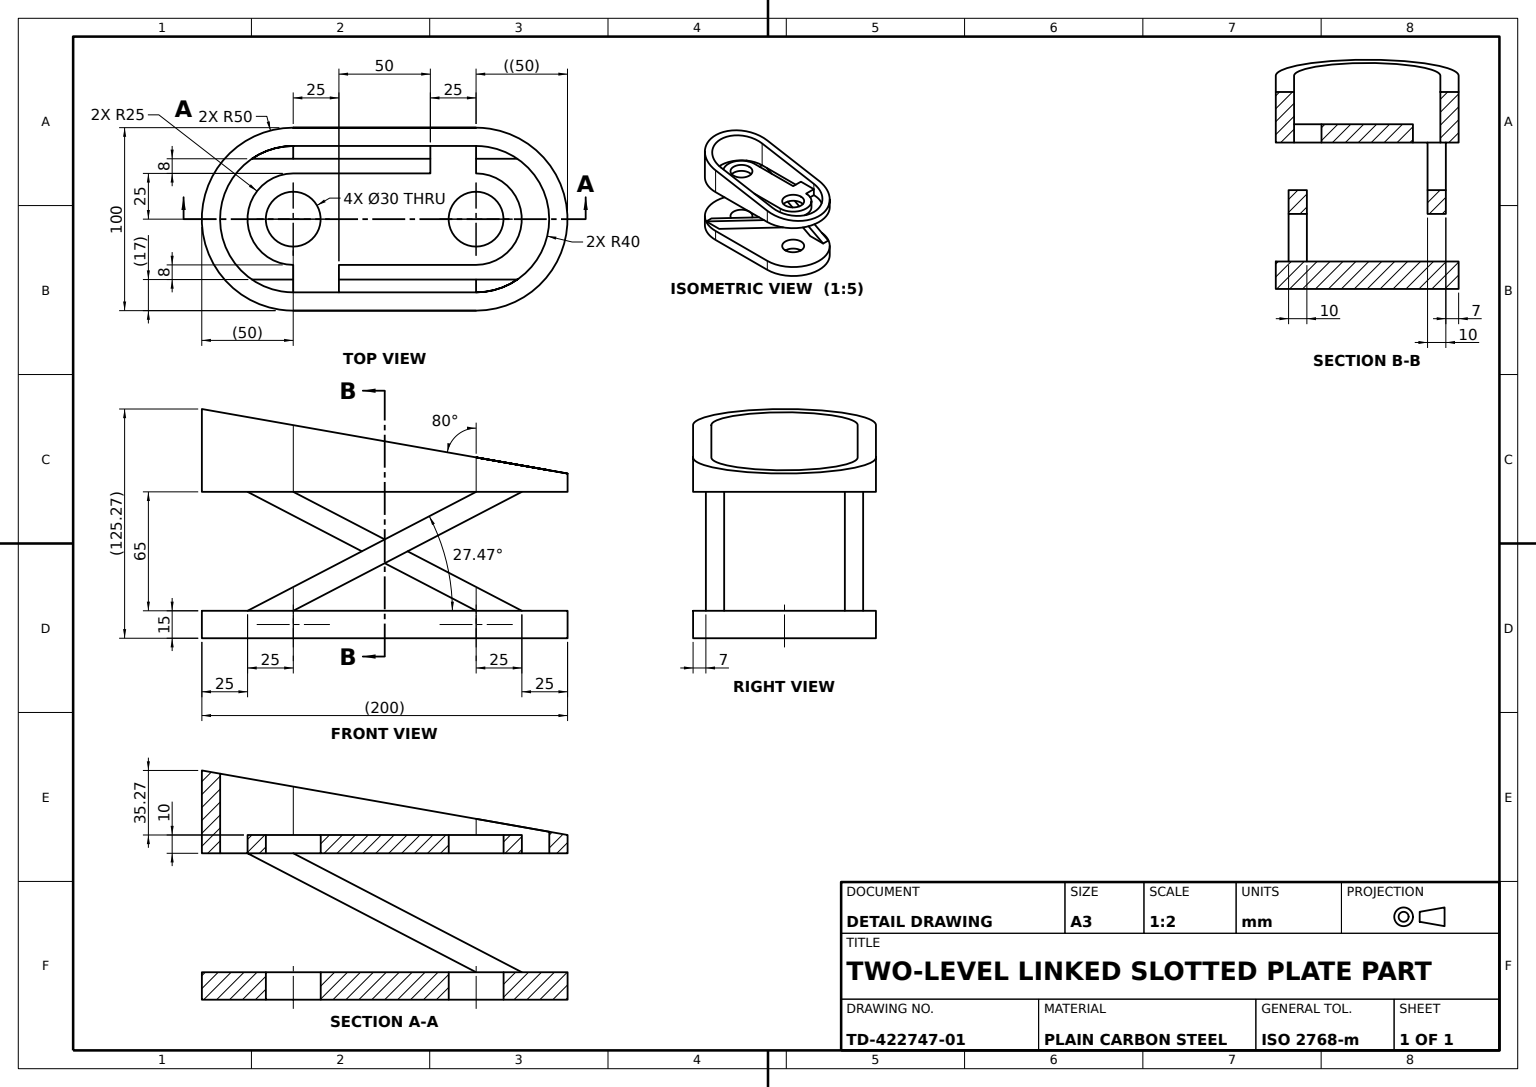
from build123d import *

# Parameters (mm, degrees)
BASE_PLATE_DEPTH         = 15
UPPER_PLATE_DEPTH        = 10
LOOP_WALL_DEPTH          = 50
LOOP_WALL_DEPTH_BACK     = 10
WALL_OPENING_CUT_DEPTH   = 160
TAB_SKETCH_W             = 25
TAB_SKETCH_H             = 10
TAB_DEPTH                = 20
GUIDE_RAIL_1_DEPTH       = 7
GUIDE_RAIL_1_DEPTH_BACK  = 3
GUIDE_RAIL_2_DEPTH       = 7
GUIDE_RAIL_2_DEPTH_BACK  = 3
ANGLED_TRIM_CUT_SKETCH_R = 15
ANGLED_TRIM_CUT_DEPTH    = 133.5


with BuildPart() as part:
    # Base Plate Sketch → Base Plate (new body)
    with BuildSketch(Plane(origin=(0, 0, 0), x_dir=(1, 0, 0), z_dir=(0, 1, 0))):
        with BuildLine():
            Line((-50, 50), (50, 50))
            ThreePointArc((50, 50), (100, 0), (50, -50))
            Line((50, -50), (-50, -50))
            ThreePointArc((-50, -50), (-100, 0), (-50, 50))
        make_face()
    extrude(amount=BASE_PLATE_DEPTH)



with BuildPart() as body_2:
    # Upper Plate Sketch → Upper Plate (new body)
    with BuildSketch(Plane(origin=(0, 80, 0), x_dir=(1, 0, 0), z_dir=(0, 1, 0))):
        with BuildLine():
            Line((50, 50), (25, 50))
            Line((25, 50), (25, 25))
            Line((25, 25), (-50, 25))
            ThreePointArc((-50, 25), (-75, 0), (-50, -25))
            Line((-50, -25), (50, -25))
            ThreePointArc((50, -25), (75, 0), (50, 25))
            Line((50, 25), (50, 50))
        make_face()
    extrude(amount=UPPER_PLATE_DEPTH)

    # Loop Wall Sketch → Loop Wall (add, two sides: drawn at the far end of the back side and taken through both)
    with BuildSketch(Plane(origin=(0, 90, 0), x_dir=(1, 0, 0), z_dir=(0, 1, 0)).offset(-LOOP_WALL_DEPTH_BACK)):
        with BuildLine():
            Line((-50, 50), (50, 50))
            ThreePointArc((50, 50), (100, 0), (50, -50))
            Line((50, -50), (-50, -50))
            ThreePointArc((-50, -50), (-100, 0), (-50, 50))
        make_face()
        with BuildLine():
            Line((-50, 40), (50, 40))
            ThreePointArc((50, 40), (90, 0), (50, -40))
            Line((50, -40), (-50, -40))
            ThreePointArc((-50, -40), (-90, 0), (-50, 40))
        make_face(mode=Mode.SUBTRACT)
    extrude(amount=LOOP_WALL_DEPTH + LOOP_WALL_DEPTH_BACK)

    # Wall Opening Cut Sketch → Wall Opening Cut (cut, symmetric)
    with BuildSketch(Plane.XY.offset(50)):
        Polygon((100, 90), (-100, 125.265396142), (-100, 140), (100, 140), align=None)
    extrude(amount=WALL_OPENING_CUT_DEPTH, both=True, mode=Mode.SUBTRACT)

    # Tab Sketch → Tab (add)
    with BuildSketch(Plane.XY.offset(25)):
        with Locations((-37.5, 85)):
            Rectangle(TAB_SKETCH_W, TAB_SKETCH_H)
    extrude(amount=TAB_DEPTH)


with BuildPart() as part_1:
    add(part.part)

    add(body_2.part)  # Guide Rail 1 merges body 2
    # Guide Rail 1 Sketch → Guide Rail 1 (add, two sides: drawn at the far end of the back side and taken through both)
    with BuildSketch(Plane.XY.offset(-40).offset(-GUIDE_RAIL_1_DEPTH_BACK)):
        Polygon((50, 15), (75, 15), (-50, 80), (-75, 80), align=None)
    extrude(amount=GUIDE_RAIL_1_DEPTH + GUIDE_RAIL_1_DEPTH_BACK)

    # Guide Rail 2 Sketch → Guide Rail 2 (add, two sides: drawn at the far end of the back side and taken through both)
    with BuildSketch(Plane(origin=(0, 0, 40), x_dir=(-1, 0, 0), z_dir=(0, 0, -1)).offset(-GUIDE_RAIL_2_DEPTH_BACK)):
        Polygon((50, 15), (75, 15), (-50, 80), (-75, 80), align=None)
    extrude(amount=GUIDE_RAIL_2_DEPTH + GUIDE_RAIL_2_DEPTH_BACK)

    # Angled Trim Cut Sketch → Angled Trim Cut (cut, symmetric)
    with BuildSketch(Plane(origin=(0, 15, 0), x_dir=(1, 0, 0), z_dir=(0, 1, 0))):
        with Locations(Location((-50, 0, 0), (0, 0, 270))):
            Circle(ANGLED_TRIM_CUT_SKETCH_R)
        with Locations(Location((50, 0, 0), (0, 0, 270))):
            Circle(ANGLED_TRIM_CUT_SKETCH_R)
    extrude(amount=ANGLED_TRIM_CUT_DEPTH, both=True, mode=Mode.SUBTRACT)


solid = part_1.part
